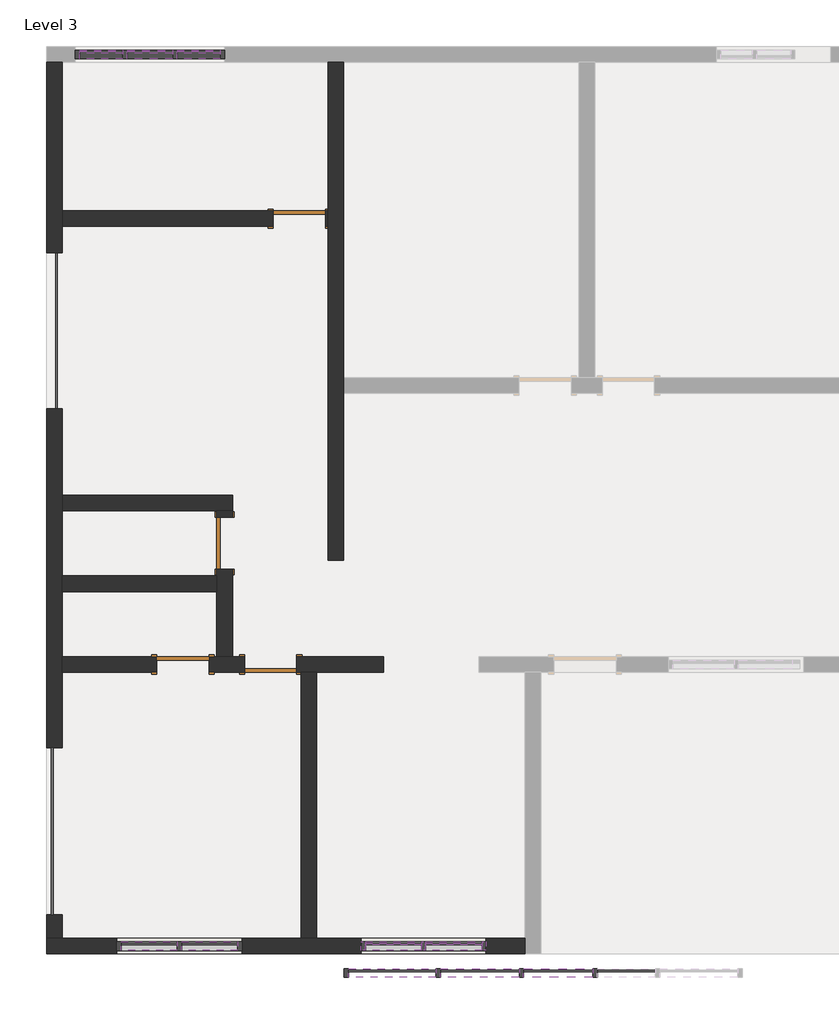
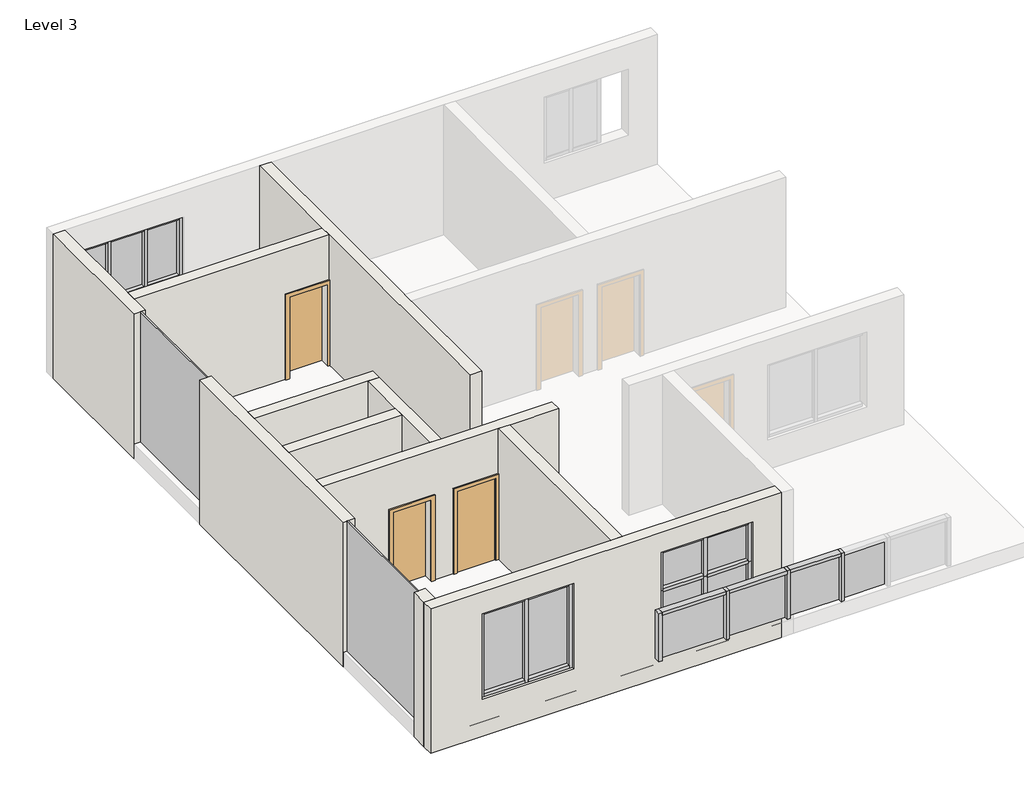
# One storey, part 1 of 2: 36 members, 15 plates, 9 walls, 4 doors.
"""IFC4 building model written with IfcOpenShell, lengths in millimetres."""

from ifc_helpers import new_model, si_unit, frame, origin, place, context, project, spatial, polyline, outline, extrude, faceted_brep, transform, mapped, element, save
from components import door_a1484949, door_85036156, member_c17f1be2, member_ad567e07, member_7f909d8d, member_1a5c3ae3, member_a88312ef, member_3e91fb70, member_7bbb9eab, member_c60babaf, member_5095b95d, member_5a9e6520, member_cba00588, member_d7472725, member_77514b12, member_7dabcdc2, member_870cb0cc, system_panel_glazed_9d4ca976, system_panel_glazed_c60cfc80, system_panel_glazed_61b33e5d, system_panel_glazed_d181f412, system_panel_glazed_8adc4deb, system_panel_glazed_f90b12a9, system_panel_glazed_bf93abc5, system_panel_glazed_f13871fb, system_panel_glazed_bbd5fb98, system_panel_glazed_1e141fc7

model = new_model("IFC4")

# Units and contexts
model_context = context("Model", 3, world=origin())
ifc_project = project(units=[si_unit("LENGTHUNIT", "METRE", prefix="MILLI")], contexts=[model_context])

# Site, building, storey
site = spatial("IfcSite", under=ifc_project)
building = spatial("IfcBuilding", under=site)
storey = spatial("IfcBuildingStorey", under=building, Name="Level 3", Elevation=6096.0)

# Doors
placement = place(None, origin())
door_shape = door_a1484949(model_context)
element("IfcDoor", 1, ObjectType="Single-Flush : 30\" x 80\"", at=placement, inside=storey, context=model_context, shape_type="MappedRepresentation", body=[
    mapped(door_shape, transform((-18291.691855, -9625.0538163, 6096.0), x_axis=(1.0, 0.0, 0.0), y_axis=(0.0, 1.0, 0.0), z_axis=(0.0, 0.0, 1.0))),
])
element("IfcDoor", 2, ObjectType="Single-Flush : 30\" x 80\"", at=placement, inside=storey, context=model_context, shape_type="MappedRepresentation", body=[
    mapped(door_shape, transform((-16589.891855, -3109.9538163, 6096.0), x_axis=(1.0, 0.0, 0.0), y_axis=(0.0, 1.0, 0.0), z_axis=(0.0, 0.0, 1.0))),
])
door_2_shape = door_85036156(model_context)
element("IfcDoor", 3, ObjectType="Single-Flush : 30\" x 80\"", at=placement, inside=storey, context=model_context, shape_type="MappedRepresentation", body=[
    mapped(door_2_shape, transform((-17008.991855, -9625.0538163, 6096.0), x_axis=(1.0, 0.0, 0.0), y_axis=(0.0, 1.0, 0.0), z_axis=(0.0, 0.0, 1.0))),
])
element("IfcDoor", 4, ObjectType="Single-Flush : 30\" x 80\"", at=placement, inside=storey, context=model_context, shape_type="MappedRepresentation", body=[
    mapped(door_2_shape, transform((-17682.091855, -7853.4038163, 6096.0), x_axis=(0.0, -1.0, 0.0), y_axis=(1.0, 0.0, 0.0), z_axis=(0.0, 0.0, 1.0))),
])

# Members
member_shape = member_c17f1be2(model_context)
element("IfcMember", 5, ObjectType="Rectangular Mullion : 2.5\" x 5\" rectangular", at=placement, inside=storey, context=model_context, shape_type="MappedRepresentation", body=[
    mapped(member_shape, transform((-14805.541855, -13739.8538163, 8725.3928177), x_axis=(0.0, 0.0, 1.0), y_axis=(0.0, -1.0, 0.0), z_axis=(1.0, 0.0, 0.0))),
])
element("IfcMember", 6, ObjectType="Rectangular Mullion : 2.5\" x 5\" rectangular", at=placement, inside=storey, context=model_context, shape_type="MappedRepresentation", body=[
    mapped(member_shape, transform((-13922.891855, -13739.8538163, 8725.3928177), x_axis=(0.0, 0.0, 1.0), y_axis=(0.0, -1.0, 0.0), z_axis=(1.0, 0.0, 0.0))),
])
element("IfcMember", 7, ObjectType="Rectangular Mullion : 2.5\" x 5\" rectangular", at=placement, inside=storey, context=model_context, shape_type="MappedRepresentation", body=[
    mapped(member_shape, transform((-18374.241855, -13739.8538163, 8676.8631794), x_axis=(0.0, 0.0, 1.0), y_axis=(0.0, -1.0, 0.0), z_axis=(1.0, 0.0, 0.0))),
])
element("IfcMember", 8, ObjectType="Rectangular Mullion : 2.5\" x 5\" rectangular", at=placement, inside=storey, context=model_context, shape_type="MappedRepresentation", body=[
    mapped(member_shape, transform((-17491.591855, -13739.8538163, 8676.8631794), x_axis=(0.0, 0.0, 1.0), y_axis=(0.0, -1.0, 0.0), z_axis=(1.0, 0.0, 0.0))),
])
member_2_shape = member_ad567e07(model_context)
element("IfcMember", 9, ObjectType="Rectangular Mullion : 2.5\" x 5\" rectangular", at=placement, inside=storey, context=model_context, shape_type="MappedRepresentation", body=[
    mapped(member_2_shape, transform((-13922.891855, -13739.8538163, 7870.5495936), x_axis=(0.0, 0.0, 1.0), y_axis=(0.0, -1.0, 0.0), z_axis=(1.0, 0.0, 0.0))),
])
element("IfcMember", 10, ObjectType="Rectangular Mullion : 2.5\" x 5\" rectangular", at=placement, inside=storey, context=model_context, shape_type="MappedRepresentation", body=[
    mapped(member_2_shape, transform((-14805.541855, -13739.8538163, 7870.5495936), x_axis=(0.0, 0.0, 1.0), y_axis=(0.0, -1.0, 0.0), z_axis=(1.0, 0.0, 0.0))),
])
element("IfcMember", 11, ObjectType="Rectangular Mullion : 2.5\" x 5\" rectangular", at=placement, inside=storey, context=model_context, shape_type="MappedRepresentation", body=[
    mapped(member_shape, transform((-14742.041855, -13739.8538163, 7015.7063696), x_axis=(0.0, 0.0, -1.0), y_axis=(0.0, -1.0, 0.0), z_axis=(-1.0, 0.0, 0.0))),
])
element("IfcMember", 12, ObjectType="Rectangular Mullion : 2.5\" x 5\" rectangular", at=placement, inside=storey, context=model_context, shape_type="MappedRepresentation", body=[
    mapped(member_shape, transform((-15624.691855, -13739.8538163, 7015.7063696), x_axis=(0.0, 0.0, -1.0), y_axis=(0.0, -1.0, 0.0), z_axis=(-1.0, 0.0, 0.0))),
])
element("IfcMember", 13, ObjectType="Rectangular Mullion : 2.5\" x 5\" rectangular", at=placement, inside=storey, context=model_context, shape_type="MappedRepresentation", body=[
    mapped(member_shape, transform((-18310.741855, -13739.8538163, 6875.7032327), x_axis=(0.0, 0.0, -1.0), y_axis=(0.0, -1.0, 0.0), z_axis=(-1.0, 0.0, 0.0))),
])
element("IfcMember", 14, ObjectType="Rectangular Mullion : 2.5\" x 5\" rectangular", at=placement, inside=storey, context=model_context, shape_type="MappedRepresentation", body=[
    mapped(member_shape, transform((-19193.391855, -13739.8538163, 6875.7032327), x_axis=(0.0, 0.0, -1.0), y_axis=(0.0, -1.0, 0.0), z_axis=(-1.0, 0.0, 0.0))),
])
member_3_shape = member_7f909d8d(model_context)
element("IfcMember", 15, ObjectType="Rectangular Mullion : 2.5\" x 5\" rectangular", at=placement, inside=storey, context=model_context, shape_type="MappedRepresentation", body=[
    mapped(member_3_shape, transform((-19170.1085217, -709.6538163, 8591.2496538), x_axis=(0.0, 0.0, 1.0), y_axis=(0.0, -1.0, 0.0), z_axis=(1.0, 0.0, 0.0))),
])
element("IfcMember", 16, ObjectType="Rectangular Mullion : 2.5\" x 5\" rectangular", at=placement, inside=storey, context=model_context, shape_type="MappedRepresentation", body=[
    mapped(member_3_shape, transform((-17745.591855, -709.6538163, 8591.2496538), x_axis=(0.0, 0.0, 1.0), y_axis=(0.0, -1.0, 0.0), z_axis=(1.0, 0.0, 0.0))),
])
member_4_shape = member_1a5c3ae3(model_context)
element("IfcMember", 17, ObjectType="Rectangular Mullion : 2.5\" x 5\" rectangular", at=placement, inside=storey, context=model_context, shape_type="MappedRepresentation", body=[
    mapped(member_4_shape, transform((-18441.9751883, -709.6538163, 8591.2496538), x_axis=(0.0, 0.0, 1.0), y_axis=(0.0, -1.0, 0.0), z_axis=(1.0, 0.0, 0.0))),
])
member_5_shape = member_a88312ef(model_context)
element("IfcMember", 18, ObjectType="Rectangular Mullion : 2.5\" x 5\" rectangular", at=placement, inside=storey, context=model_context, shape_type="MappedRepresentation", body=[
    mapped(member_5_shape, transform((-19138.3585217, -709.6538163, 7292.9915007), x_axis=(1.0, 0.0, 0.0), y_axis=(0.0, -1.0, 0.0), z_axis=(0.0, 0.0, -1.0))),
])
element("IfcMember", 19, ObjectType="Rectangular Mullion : 2.5\" x 5\" rectangular", at=placement, inside=storey, context=model_context, shape_type="MappedRepresentation", body=[
    mapped(member_5_shape, transform((-18410.2251883, -709.6538163, 7292.9915007), x_axis=(1.0, 0.0, 0.0), y_axis=(0.0, -1.0, 0.0), z_axis=(0.0, 0.0, -1.0))),
])
element("IfcMember", 20, ObjectType="Rectangular Mullion : 2.5\" x 5\" rectangular", at=placement, inside=storey, context=model_context, shape_type="MappedRepresentation", body=[
    mapped(member_4_shape, transform((-19106.6085217, -709.6538163, 7292.9915007), x_axis=(0.0, 0.0, -1.0), y_axis=(0.0, -1.0, 0.0), z_axis=(-1.0, 0.0, 0.0))),
])
element("IfcMember", 21, ObjectType="Rectangular Mullion : 2.5\" x 5\" rectangular", at=placement, inside=storey, context=model_context, shape_type="MappedRepresentation", body=[
    mapped(member_3_shape, transform((-18378.4751883, -709.6538163, 7292.9915007), x_axis=(0.0, 0.0, -1.0), y_axis=(0.0, -1.0, 0.0), z_axis=(-1.0, 0.0, 0.0))),
])
element("IfcMember", 22, ObjectType="Rectangular Mullion : 2.5\" x 5\" rectangular", at=placement, inside=storey, context=model_context, shape_type="MappedRepresentation", body=[
    mapped(member_3_shape, transform((-19802.991855, -709.6538163, 7292.9915007), x_axis=(0.0, 0.0, -1.0), y_axis=(0.0, -1.0, 0.0), z_axis=(-1.0, 0.0, 0.0))),
])
member_6_shape = member_3e91fb70(model_context)
element("IfcMember", 23, ObjectType="Rectangular Mullion : 2.5\" x 5\" rectangular", at=placement, inside=storey, context=model_context, shape_type="MappedRepresentation", body=[
    mapped(member_6_shape, transform((-19866.491855, -709.6538163, 8591.2496538), x_axis=(-1.0, 0.0, 0.0), y_axis=(0.0, -1.0, 0.0), z_axis=(0.0, 0.0, 1.0))),
])
element("IfcMember", 24, ObjectType="Rectangular Mullion : 2.5\" x 5\" rectangular", at=placement, inside=storey, context=model_context, shape_type="MappedRepresentation", body=[
    mapped(member_6_shape, transform((-17682.091855, -709.6538163, 7292.9915007), x_axis=(1.0, 0.0, 0.0), y_axis=(0.0, -1.0, 0.0), z_axis=(0.0, 0.0, -1.0))),
])
member_7_shape = member_7bbb9eab(model_context)
element("IfcMember", 25, ObjectType="Rectangular Mullion : 2.5\" x 5\" rectangular", at=placement, inside=storey, context=model_context, shape_type="MappedRepresentation", body=[
    mapped(member_7_shape, transform((-14773.791855, -13739.8538163, 7870.5495936), x_axis=(1.0, 0.0, 0.0), y_axis=(0.0, -1.0, 0.0), z_axis=(0.0, 0.0, -1.0))),
])
member_8_shape = member_c60babaf(model_context)
element("IfcMember", 26, ObjectType="Rectangular Mullion : 2.5\" x 5\" rectangular", at=placement, inside=storey, context=model_context, shape_type="MappedRepresentation", body=[
    mapped(member_8_shape, transform((-15688.191855, -13739.8538163, 8725.3928177), x_axis=(-1.0, 0.0, 0.0), y_axis=(0.0, -1.0, 0.0), z_axis=(0.0, 0.0, 1.0))),
])
element("IfcMember", 27, ObjectType="Rectangular Mullion : 2.5\" x 5\" rectangular", at=placement, inside=storey, context=model_context, shape_type="MappedRepresentation", body=[
    mapped(member_7_shape, transform((-14773.791855, -13739.8538163, 7015.7063696), x_axis=(1.0, 0.0, 0.0), y_axis=(0.0, -1.0, 0.0), z_axis=(0.0, 0.0, -1.0))),
])
element("IfcMember", 28, ObjectType="Rectangular Mullion : 2.5\" x 5\" rectangular", at=placement, inside=storey, context=model_context, shape_type="MappedRepresentation", body=[
    mapped(member_8_shape, transform((-15688.191855, -13739.8538163, 7870.5495936), x_axis=(-1.0, 0.0, 0.0), y_axis=(0.0, -1.0, 0.0), z_axis=(0.0, 0.0, 1.0))),
])
element("IfcMember", 29, ObjectType="Rectangular Mullion : 2.5\" x 5\" rectangular", at=placement, inside=storey, context=model_context, shape_type="MappedRepresentation", body=[
    mapped(member_8_shape, transform((-13859.391855, -13739.8538163, 7870.5495936), x_axis=(1.0, 0.0, 0.0), y_axis=(0.0, -1.0, 0.0), z_axis=(0.0, 0.0, -1.0))),
])
element("IfcMember", 30, ObjectType="Rectangular Mullion : 2.5\" x 5\" rectangular", at=placement, inside=storey, context=model_context, shape_type="MappedRepresentation", body=[
    mapped(member_8_shape, transform((-13859.391855, -13739.8538163, 7015.7063696), x_axis=(1.0, 0.0, 0.0), y_axis=(0.0, -1.0, 0.0), z_axis=(0.0, 0.0, -1.0))),
])
member_9_shape = member_5095b95d(model_context)
element("IfcMember", 31, ObjectType="Rectangular Mullion : 2.5\" x 5\" rectangular", at=placement, inside=storey, context=model_context, shape_type="MappedRepresentation", body=[
    mapped(member_9_shape, transform((-18342.491855, -13739.8538163, 6875.7032327), x_axis=(1.0, 0.0, 0.0), y_axis=(0.0, -1.0, 0.0), z_axis=(0.0, 0.0, -1.0))),
])
member_10_shape = member_5a9e6520(model_context)
element("IfcMember", 32, ObjectType="Rectangular Mullion : 2.5\" x 5\" rectangular", at=placement, inside=storey, context=model_context, shape_type="MappedRepresentation", body=[
    mapped(member_10_shape, transform((-17428.091855, -13739.8538163, 6875.7032327), x_axis=(1.0, 0.0, 0.0), y_axis=(0.0, -1.0, 0.0), z_axis=(0.0, 0.0, -1.0))),
])
element("IfcMember", 33, ObjectType="Rectangular Mullion : 2.5\" x 5\" rectangular", at=placement, inside=storey, context=model_context, shape_type="MappedRepresentation", body=[
    mapped(member_10_shape, transform((-19256.891855, -13739.8538163, 8676.8631794), x_axis=(-1.0, 0.0, 0.0), y_axis=(0.0, -1.0, 0.0), z_axis=(0.0, 0.0, 1.0))),
])
member_11_shape = member_cba00588(model_context)
element("IfcMember", 34, ObjectType="Rectangular Mullion : 2.5\" x 5\" rectangular", at=placement, inside=storey, context=model_context, shape_type="MappedRepresentation", body=[
    mapped(member_11_shape, transform((-14592.3932214, -14133.5538163, 7725.553622), x_axis=(0.0, 0.0, 1.0), y_axis=(0.0, -1.0, 0.0), z_axis=(1.0, 0.0, 0.0))),
])
member_12_shape = member_d7472725(model_context)
element("IfcMember", 35, ObjectType="Rectangular Mullion : 2.5\" x 5\" rectangular", at=placement, inside=storey, context=model_context, shape_type="MappedRepresentation", body=[
    mapped(member_12_shape, transform((-13373.1932214, -14133.5538163, 7725.553622), x_axis=(0.0, 0.0, 1.0), y_axis=(0.0, -1.0, 0.0), z_axis=(1.0, 0.0, 0.0))),
])
member_13_shape = member_77514b12(model_context)
element("IfcMember", 36, ObjectType="Rectangular Mullion : 2.5\" x 5\" rectangular", at=placement, inside=storey, context=model_context, shape_type="MappedRepresentation", body=[
    mapped(member_13_shape, transform((-12297.9265548, -14133.5538163, 7725.553622), x_axis=(0.0, 0.0, 1.0), y_axis=(0.0, -1.0, 0.0), z_axis=(1.0, 0.0, 0.0))),
])
member_14_shape = member_7dabcdc2(model_context)
element("IfcMember", 37, ObjectType="Rectangular Mullion : 2.5\" x 5\" rectangular", at=placement, inside=storey, context=model_context, shape_type="MappedRepresentation", body=[
    mapped(member_14_shape, transform((-14560.6432214, -14133.5538163, 6705.6), x_axis=(1.0, 0.0, 0.0), y_axis=(0.0, -1.0, 0.0), z_axis=(0.0, 0.0, -1.0))),
])
element("IfcMember", 38, ObjectType="Rectangular Mullion : 2.5\" x 5\" rectangular", at=placement, inside=storey, context=model_context, shape_type="MappedRepresentation", body=[
    mapped(member_14_shape, transform((-13341.4432214, -14133.5538163, 6705.6), x_axis=(1.0, 0.0, 0.0), y_axis=(0.0, -1.0, 0.0), z_axis=(0.0, 0.0, -1.0))),
])
element("IfcMember", 39, ObjectType="Rectangular Mullion : 2.5\" x 5\" rectangular", at=placement, inside=storey, context=model_context, shape_type="MappedRepresentation", body=[
    mapped(member_14_shape, transform((-12266.1765548, -14133.5538163, 6705.6), x_axis=(1.0, 0.0, 0.0), y_axis=(0.0, -1.0, 0.0), z_axis=(0.0, 0.0, -1.0))),
])
member_15_shape = member_870cb0cc(model_context)
element("IfcMember", 40, ObjectType="Rectangular Mullion : 2.5\" x 5\" rectangular", at=placement, inside=storey, context=model_context, shape_type="MappedRepresentation", body=[
    mapped(member_15_shape, transform((-15932.2432214, -14133.5538163, 7725.553622), x_axis=(-1.0, 0.0, 0.0), y_axis=(0.0, -1.0, 0.0), z_axis=(0.0, 0.0, 1.0))),
])

# Plates
system_panel_glazed_shape = system_panel_glazed_9d4ca976(model_context)
element("IfcPlate", 41, ObjectType="System Panel : Glazed", at=placement, inside=storey, context=model_context, shape_type="MappedRepresentation", body=[
    mapped(system_panel_glazed_shape, transform((-20171.291855, -4748.2538163, 6096.0), x_axis=(0.0, -1.0, 0.0), y_axis=(1.0, 0.0, 0.0), z_axis=(0.0, 0.0, 1.0))),
])
system_panel_glazed_2_shape = system_panel_glazed_c60cfc80(model_context)
element("IfcPlate", 42, ObjectType="System Panel : Glazed", at=placement, inside=storey, context=model_context, shape_type="MappedRepresentation", body=[
    mapped(system_panel_glazed_2_shape, transform((-20171.291855, -12063.4538163, 6096.0), x_axis=(0.0, 1.0, 0.0), y_axis=(-1.0, 0.0, 0.0), z_axis=(0.0, 0.0, 1.0))),
])
system_panel_glazed_3_shape = system_panel_glazed_61b33e5d(model_context)
element("IfcPlate", 43, ObjectType="System Panel : Glazed", at=placement, inside=storey, context=model_context, shape_type="MappedRepresentation", body=[
    mapped(system_panel_glazed_3_shape, transform((-19486.5501883, -709.6538163, 7356.4915007), x_axis=(1.0, 0.0, 0.0), y_axis=(0.0, 1.0, 0.0), z_axis=(0.0, 0.0, 1.0))),
])
element("IfcPlate", 44, ObjectType="System Panel : Glazed", at=placement, inside=storey, context=model_context, shape_type="MappedRepresentation", body=[
    mapped(system_panel_glazed_3_shape, transform((-18062.0335217, -709.6538163, 7356.4915007), x_axis=(1.0, 0.0, 0.0), y_axis=(0.0, 1.0, 0.0), z_axis=(0.0, 0.0, 1.0))),
])
system_panel_glazed_4_shape = system_panel_glazed_d181f412(model_context)
element("IfcPlate", 45, ObjectType="System Panel : Glazed", at=placement, inside=storey, context=model_context, shape_type="MappedRepresentation", body=[
    mapped(system_panel_glazed_4_shape, transform((-18774.291855, -709.6538163, 7356.4915007), x_axis=(1.0, 0.0, 0.0), y_axis=(0.0, 1.0, 0.0), z_axis=(0.0, 0.0, 1.0))),
])
system_panel_glazed_5_shape = system_panel_glazed_8adc4deb(model_context)
element("IfcPlate", 46, ObjectType="System Panel : Glazed", at=placement, inside=storey, context=model_context, shape_type="MappedRepresentation", body=[
    mapped(system_panel_glazed_5_shape, transform((-15215.116855, -13739.8538163, 7079.2063696), x_axis=(1.0, 0.0, 0.0), y_axis=(0.0, 1.0, 0.0), z_axis=(0.0, 0.0, 1.0))),
])
element("IfcPlate", 47, ObjectType="System Panel : Glazed", at=placement, inside=storey, context=model_context, shape_type="MappedRepresentation", body=[
    mapped(system_panel_glazed_5_shape, transform((-14332.466855, -13739.8538163, 7079.2063696), x_axis=(1.0, 0.0, 0.0), y_axis=(0.0, 1.0, 0.0), z_axis=(0.0, 0.0, 1.0))),
])
element("IfcPlate", 48, ObjectType="System Panel : Glazed", at=placement, inside=storey, context=model_context, shape_type="MappedRepresentation", body=[
    mapped(system_panel_glazed_5_shape, transform((-15215.116855, -13739.8538163, 7902.2995936), x_axis=(1.0, 0.0, 0.0), y_axis=(0.0, 1.0, 0.0), z_axis=(0.0, 0.0, 1.0))),
])
element("IfcPlate", 49, ObjectType="System Panel : Glazed", at=placement, inside=storey, context=model_context, shape_type="MappedRepresentation", body=[
    mapped(system_panel_glazed_5_shape, transform((-14332.466855, -13739.8538163, 7902.2995936), x_axis=(1.0, 0.0, 0.0), y_axis=(0.0, 1.0, 0.0), z_axis=(0.0, 0.0, 1.0))),
])
system_panel_glazed_6_shape = system_panel_glazed_f90b12a9(model_context)
element("IfcPlate", 50, ObjectType="System Panel : Glazed", at=placement, inside=storey, context=model_context, shape_type="MappedRepresentation", body=[
    mapped(system_panel_glazed_6_shape, transform((-18783.816855, -13739.8538163, 6939.2032327), x_axis=(1.0, 0.0, 0.0), y_axis=(0.0, 1.0, 0.0), z_axis=(0.0, 0.0, 1.0))),
])
element("IfcPlate", 51, ObjectType="System Panel : Glazed", at=placement, inside=storey, context=model_context, shape_type="MappedRepresentation", body=[
    mapped(system_panel_glazed_6_shape, transform((-17901.166855, -13739.8538163, 6939.2032327), x_axis=(1.0, 0.0, 0.0), y_axis=(0.0, 1.0, 0.0), z_axis=(0.0, 0.0, 1.0))),
])
system_panel_glazed_7_shape = system_panel_glazed_bf93abc5(model_context)
element("IfcPlate", 52, ObjectType="System Panel : Glazed", at=placement, inside=storey, context=model_context, shape_type="MappedRepresentation", body=[
    mapped(system_panel_glazed_7_shape, transform((-15230.5682214, -14133.5538163, 6705.6), x_axis=(1.0, 0.0, 0.0), y_axis=(0.0, 1.0, 0.0), z_axis=(0.0, 0.0, 1.0))),
])
system_panel_glazed_8_shape = system_panel_glazed_f13871fb(model_context)
element("IfcPlate", 53, ObjectType="System Panel : Glazed", at=placement, inside=storey, context=model_context, shape_type="MappedRepresentation", body=[
    mapped(system_panel_glazed_8_shape, transform((-13951.0432214, -14133.5538163, 6705.6), x_axis=(1.0, 0.0, 0.0), y_axis=(0.0, 1.0, 0.0), z_axis=(0.0, 0.0, 1.0))),
])
system_panel_glazed_9_shape = system_panel_glazed_bbd5fb98(model_context)
element("IfcPlate", 54, ObjectType="System Panel : Glazed", at=placement, inside=storey, context=model_context, shape_type="MappedRepresentation", body=[
    mapped(system_panel_glazed_9_shape, transform((-12803.8098881, -14133.5538163, 6705.6), x_axis=(1.0, 0.0, 0.0), y_axis=(0.0, 1.0, 0.0), z_axis=(0.0, 0.0, 1.0))),
])
system_panel_glazed_10_shape = system_panel_glazed_1e141fc7(model_context)
element("IfcPlate", 55, ObjectType="System Panel : Glazed", at=placement, inside=storey, context=model_context, shape_type="MappedRepresentation", body=[
    mapped(system_panel_glazed_10_shape, transform((-11808.9765548, -14133.5538163, 6705.6), x_axis=(1.0, 0.0, 0.0), y_axis=(0.0, 1.0, 0.0), z_axis=(0.0, 0.0, 1.0))),
])

# Walls
element("IfcWall", 56, ObjectType="9\"", at=placement, inside=storey, context=model_context, shape_type="Brep", body=[
    faceted_brep([(-13287.891855, -13625.5538163, 6096.0), (-16335.891855, -13625.5538163, 6096.0), (-16564.491855, -13625.5538163, 6096.0), (-20056.991855, -13625.5538163, 6096.0), (-20285.591855, -13625.5538163, 6096.0), (-20285.591855, -13625.5538163, 9144.0), (-20056.991855, -13625.5538163, 9144.0), (-16564.491855, -13625.5538163, 9144.0), (-16335.891855, -13625.5538163, 9144.0), (-13287.891855, -13625.5538163, 9144.0), (-15688.191855, -13625.5538163, 8725.3928177), (-15688.191855, -13625.5538163, 7015.7063696), (-13859.391855, -13625.5538163, 7015.7063696), (-13859.391855, -13625.5538163, 8725.3928177), (-19256.891855, -13625.5538163, 8676.8631794), (-19256.891855, -13625.5538163, 6875.7032327), (-17428.091855, -13625.5538163, 6875.7032327), (-17428.091855, -13625.5538163, 8676.8631794), (-20285.591855, -13854.1538163, 6096.0), (-13287.891855, -13854.1538163, 6096.0), (-13287.891855, -13854.1538163, 9144.0), (-20285.591855, -13854.1538163, 9144.0), (-15688.191855, -13854.1538163, 7015.7063696), (-15688.191855, -13854.1538163, 8725.3928177), (-13859.391855, -13854.1538163, 8725.3928177), (-13859.391855, -13854.1538163, 7015.7063696), (-19256.891855, -13854.1538163, 6875.7032327), (-19256.891855, -13854.1538163, 8676.8631794), (-17428.091855, -13854.1538163, 8676.8631794), (-17428.091855, -13854.1538163, 6875.7032327)], [[[0, 1, 2, 3, 4, 5, 6, 7, 8, 9], [10, 11, 12, 13], [14, 15, 16, 17]], [[18, 19, 20, 21], [22, 23, 24, 25], [26, 27, 28, 29]], [[4, 3, 2, 1, 0, 19, 18]], [[9, 8, 7, 6, 5, 21, 20]], [[0, 9, 20, 19]], [[5, 4, 18, 21]], [[10, 23, 22, 11]], [[23, 10, 13, 24]], [[24, 13, 12, 25]], [[11, 22, 25, 12]], [[26, 15, 14, 27]], [[27, 14, 17, 28]], [[28, 17, 16, 29]], [[15, 26, 29, 16]]]),
])
element("IfcWall", 57, ObjectType="9\"", at=placement, inside=storey, context=model_context, shape_type="Brep", body=[
    faceted_brep([(-20056.991855, -13625.5538163, 9144.0), (-20056.991855, -13625.5538163, 6096.0), (-20056.991855, -13282.6538163, 6096.0), (-20056.991855, -13282.6538163, 9144.0), (-20285.591855, -13625.5538163, 6096.0), (-20285.591855, -13625.5538163, 9144.0), (-20285.591855, -13282.6538163, 9144.0), (-20285.591855, -13282.6538163, 6096.0)], [[[0, 1, 2, 3]], [[4, 5, 6, 7]], [[1, 4, 7, 2]], [[5, 0, 3, 6]], [[1, 0, 5, 4]], [[3, 2, 7, 6]]]),
    faceted_brep([(-20056.991855, -823.9538163, 6096.0), (-20056.991855, -823.9538163, 9144.0), (-20056.991855, -2995.6538163, 9144.0), (-20056.991855, -3224.2538163, 9144.0), (-20056.991855, -3605.2538163, 9144.0), (-20056.991855, -3605.2538163, 6096.0), (-20056.991855, -3224.2538163, 6096.0), (-20056.991855, -2995.6538163, 6096.0), (-20285.591855, -823.9538163, 9144.0), (-20285.591855, -823.9538163, 6096.0), (-20285.591855, -3605.2538163, 6096.0), (-20285.591855, -3605.2538163, 9144.0)], [[[0, 1, 2, 3, 4, 5, 6, 7]], [[8, 9, 10, 11]], [[9, 0, 7, 6, 5, 10]], [[1, 8, 11, 4, 3, 2]], [[1, 0, 9, 8]], [[5, 4, 11, 10]]]),
    faceted_brep([(-20056.991855, -5891.2538163, 6096.0), (-20056.991855, -5891.2538163, 9144.0), (-20056.991855, -7148.5538163, 9144.0), (-20056.991855, -7377.1538163, 9144.0), (-20056.991855, -8329.6538163, 9144.0), (-20056.991855, -8558.2538163, 9144.0), (-20056.991855, -9510.7538163, 9144.0), (-20056.991855, -9739.3538163, 9144.0), (-20056.991855, -10844.2538163, 9144.0), (-20056.991855, -10844.2538163, 6096.0), (-20056.991855, -9739.3538163, 6096.0), (-20056.991855, -9510.7538163, 6096.0), (-20056.991855, -8558.2538163, 6096.0), (-20056.991855, -8329.6538163, 6096.0), (-20056.991855, -7377.1538163, 6096.0), (-20056.991855, -7148.5538163, 6096.0), (-20285.591855, -5891.2538163, 9144.0), (-20285.591855, -5891.2538163, 6096.0), (-20285.591855, -10844.2538163, 6096.0), (-20285.591855, -10844.2538163, 9144.0)], [[[0, 1, 2, 3, 4, 5, 6, 7, 8, 9, 10, 11, 12, 13, 14, 15]], [[16, 17, 18, 19]], [[17, 0, 15, 14, 13, 12, 11, 10, 9, 18]], [[1, 16, 19, 8, 7, 6, 5, 4, 3, 2]], [[1, 0, 17, 16]], [[9, 8, 19, 18]]]),
])
element("IfcWall", 58, ObjectType="9\"", at=placement, inside=storey, context=model_context, shape_type="SweptSolid", body=[
    extrude(outline(polyline([(8128.0, -16208.891855), (6096.0, -16208.891855), (6096.0, -16170.791855), (9144.0, -16170.791855), (9144.0, -20056.991855), (6096.0, -20056.991855), (6096.0, -16970.891855), (8128.0, -16970.891855), (8128.0, -16208.891855)])), frame((0.0, -3224.2538163, 0.0), z_axis=(0.0, 1.0, 0.0), x_axis=(0.0, 0.0, 1.0)), (0.0, 0.0, 1.0), 228.6),
])
element("IfcWall", 59, ObjectType="9\"", at=placement, inside=storey, context=model_context, shape_type="Brep", body=[
    faceted_brep([(-15942.191855, -8101.0538163, 6096.0), (-15942.191855, -5662.6538163, 6096.0), (-15942.191855, -5434.0538163, 6096.0), (-15942.191855, -823.9538163, 6096.0), (-15942.191855, -823.9538163, 9144.0), (-15942.191855, -5434.0538163, 9144.0), (-15942.191855, -5662.6538163, 9144.0), (-15942.191855, -8101.0538163, 9144.0), (-16170.791855, -8101.0538163, 6096.0), (-16170.791855, -8101.0538163, 9144.0), (-16170.791855, -3224.2538163, 9144.0), (-16170.791855, -2995.6538163, 9144.0), (-16170.791855, -823.9538163, 9144.0), (-16170.791855, -823.9538163, 6096.0), (-16170.791855, -2995.6538163, 6096.0), (-16170.791855, -3224.2538163, 6096.0)], [[[0, 1, 2, 3, 4, 5, 6, 7]], [[8, 9, 10, 11, 12, 13, 14, 15]], [[3, 2, 1, 0, 8, 15, 14, 13]], [[7, 6, 5, 4, 12, 11, 10, 9]], [[0, 7, 9, 8]], [[4, 3, 13, 12]]]),
])
element("IfcWall", 60, ObjectType="9\"", at=placement, inside=storey, context=model_context, shape_type="SweptSolid", body=[
    extrude(outline(polyline([(-16335.891855, -9739.3538163), (-16335.891855, -13625.5538163), (-16564.491855, -13625.5538163), (-16564.491855, -9739.3538163), (-16335.891855, -9739.3538163)])), frame((0.0, 0.0, 6096.0), z_axis=(0.0, 0.0, 1.0), x_axis=(1.0, 0.0, 0.0)), (0.0, 0.0, 1.0), 3048.0),
])
element("IfcWall", 61, ObjectType="9\"", at=placement, inside=storey, context=model_context, shape_type="Brep", body=[
    faceted_brep([(-17910.691855, -9739.3538163, 8128.0), (-17910.691855, -9739.3538163, 6096.0), (-17389.991855, -9739.3538163, 6096.0), (-17389.991855, -9739.3538163, 8128.0), (-16627.991855, -9739.3538163, 8128.0), (-16627.991855, -9739.3538163, 6096.0), (-16564.491855, -9739.3538163, 6096.0), (-16335.891855, -9739.3538163, 6096.0), (-15357.991855, -9739.3538163, 6096.0), (-15357.991855, -9739.3538163, 9144.0), (-16335.891855, -9739.3538163, 9144.0), (-16564.491855, -9739.3538163, 9144.0), (-20056.991855, -9739.3538163, 9144.0), (-20056.991855, -9739.3538163, 6096.0), (-18672.691855, -9739.3538163, 6096.0), (-18672.691855, -9739.3538163, 8128.0), (-17389.991855, -9510.7538163, 6096.0), (-17567.791855, -9510.7538163, 6096.0), (-17796.391855, -9510.7538163, 6096.0), (-17910.691855, -9510.7538163, 6096.0), (-17910.691855, -9510.7538163, 8128.0), (-18672.691855, -9510.7538163, 8128.0), (-18672.691855, -9510.7538163, 6096.0), (-20056.991855, -9510.7538163, 6096.0), (-20056.991855, -9510.7538163, 9144.0), (-17796.391855, -9510.7538163, 9144.0), (-17567.791855, -9510.7538163, 9144.0), (-15357.991855, -9510.7538163, 9144.0), (-15357.991855, -9510.7538163, 6096.0), (-16627.991855, -9510.7538163, 6096.0), (-16627.991855, -9510.7538163, 8128.0), (-17389.991855, -9510.7538163, 8128.0)], [[[0, 1, 2, 3, 4, 5, 6, 7, 8, 9, 10, 11, 12, 13, 14, 15]], [[16, 17, 18, 19, 20, 21, 22, 23, 24, 25, 26, 27, 28, 29, 30, 31]], [[8, 7, 6, 5, 29, 28]], [[14, 13, 23, 22]], [[2, 1, 19, 18, 17, 16]], [[9, 8, 28, 27]], [[12, 11, 10, 9, 27, 26, 25, 24]], [[13, 12, 24, 23]], [[30, 29, 5, 4]], [[31, 30, 4, 3]], [[16, 31, 3, 2]], [[20, 19, 1, 0]], [[21, 20, 0, 15]], [[22, 21, 15, 14]]]),
])
element("IfcWall", 62, ObjectType="9\"", at=placement, inside=storey, context=model_context, shape_type="Brep", body=[
    faceted_brep([(-20056.991855, -7377.1538163, 6096.0), (-17796.391855, -7377.1538163, 6096.0), (-17567.791855, -7377.1538163, 6096.0), (-17567.791855, -7377.1538163, 9144.0), (-17796.391855, -7377.1538163, 9144.0), (-20056.991855, -7377.1538163, 9144.0), (-20056.991855, -7148.5538163, 6096.0), (-20056.991855, -7148.5538163, 9144.0), (-17567.791855, -7148.5538163, 9144.0), (-17567.791855, -7148.5538163, 6096.0)], [[[0, 1, 2, 3, 4, 5]], [[6, 7, 8, 9]], [[2, 1, 0, 6, 9]], [[5, 4, 3, 8, 7]], [[0, 5, 7, 6]], [[3, 2, 9, 8]]]),
])
element("IfcWall", 63, ObjectType="9\"", at=placement, inside=storey, context=model_context, shape_type="Brep", body=[
    faceted_brep([(-17796.391855, -8234.4038163, 8128.0), (-17796.391855, -8234.4038163, 6096.0), (-17796.391855, -8329.6538163, 6096.0), (-17796.391855, -8558.2538163, 6096.0), (-17796.391855, -9510.7538163, 6096.0), (-17796.391855, -9510.7538163, 9144.0), (-17796.391855, -8558.2538163, 9144.0), (-17796.391855, -8329.6538163, 9144.0), (-17796.391855, -7377.1538163, 9144.0), (-17796.391855, -7377.1538163, 6096.0), (-17796.391855, -7472.4038163, 6096.0), (-17796.391855, -7472.4038163, 8128.0), (-17567.791855, -9510.7538163, 6096.0), (-17567.791855, -8234.4038163, 6096.0), (-17567.791855, -8234.4038163, 8128.0), (-17567.791855, -7472.4038163, 8128.0), (-17567.791855, -7472.4038163, 6096.0), (-17567.791855, -7377.1538163, 6096.0), (-17567.791855, -7377.1538163, 9144.0), (-17567.791855, -9510.7538163, 9144.0)], [[[0, 1, 2, 3, 4, 5, 6, 7, 8, 9, 10, 11]], [[12, 13, 14, 15, 16, 17, 18, 19]], [[10, 9, 17, 16]], [[4, 3, 2, 1, 13, 12]], [[8, 7, 6, 5, 19, 18]], [[9, 8, 18, 17]], [[5, 4, 12, 19]], [[14, 13, 1, 0]], [[15, 14, 0, 11]], [[16, 15, 11, 10]]]),
])
element("IfcWall", 64, ObjectType="9\"", at=placement, inside=storey, context=model_context, shape_type="SweptSolid", body=[
    extrude(outline(polyline([(-20056.991855, -8329.6538163), (-17796.391855, -8329.6538163), (-17796.391855, -8558.2538163), (-20056.991855, -8558.2538163), (-20056.991855, -8329.6538163)])), frame((0.0, 0.0, 6096.0), z_axis=(0.0, 0.0, 1.0), x_axis=(1.0, 0.0, 0.0)), (0.0, 0.0, 1.0), 3048.0),
])

save(model, "model.ifc")

# Revit data of these elements
# Type "Single-Flush : 30\" x 80\""
#   Type Mark = "5"
#   Construction Type Id = "MDOOR"
#   Assembly Code = "C1020"
#   Analytic Construction = "Metal"
#   Thickness = 0' - 2"
#   Heat Transfer Coefficient (U) = 0.651978 BTU/(h·ft²·°F)
#   Height = 6' - 8"
#   Trim Projection Ext = 0' - 1"
#   Trim Projection Int = 0' - 1"
#   Trim Width = 0' - 3"
#   Width = 2' - 6"
#   Define Thermal Properties by = 1
#   Define Thermal Properties by = 1
#   Door Material = Door - Panel
#   Frame Material = Door - Frame
#   Visual Light Transmittance = 0
#   Solar Heat Gain Coefficient = 0
#   Function = (empty or 0)
#   Wall Closure = (empty or 0)
# Type "Rectangular Mullion : 2.5\" x 5\" rectangular"
#   built-in parameter 1007304 = 0.416667 (stored number, unit not read)
#   built-in parameter 1007301 = 0.104167 (stored number, unit not read)
#   built-in parameter 1007300 = 0.104167 (stored number, unit not read)
# Type "System Panel : Glazed"
#   Construction Type Id = "GSP4R"
#   Analytic Construction = "1/8 in Pilkington single glazing"
#   Visual Light Transmittance = 0.9
#   Solar Heat Gain Coefficient = 0.86
#   Heat Transfer Coefficient (U) = 1.18115 BTU/(h·ft²·°F)
#   Define Thermal Properties by = 1
# Type "9\""
#   Assembly Code = "B2010"
#   Layers, outside or top first: 0' - 9" no material (function 1)
# Elements 1, 2, 3, 4 (IfcDoor, "Single-Flush : 30\" x 80\"")
#   Phase Created = New Construction
#   Materials on its faces: "Door - Frame", "Door - Panel"
# Elements 5, 6, 7, 8, 9, 10, 11, 12, 13, 14, 15, 16, 17, 18, 19, 20, 21, 22, 23, 24, 25, 26, 27, 28, 29, 30, 31, 32, 33, 34, 35, 36, 37, 38, 39, 40 (IfcMember, "Rectangular Mullion : 2.5\" x 5\" rectangular")
#   Phase Created = New Construction
#   Materials on its faces: "Aluminum"
# Elements 41, 42, 43, 44, 45, 46, 47, 48, 49, 50, 51, 52, 53, 54, 55 (IfcPlate, "System Panel : Glazed")
#   Phase Created = New Construction
#   Materials on its faces: "Glass"
# Elements 56, 57, 58, 59, 60, 61, 62, 63, 64 (IfcWall, "9\"")
#   Top Offset = 0' - 0"
#   Base Offset = 0' - 0"
#   Unconnected Height = 10' - 0"
#   wall height = 10' - 0"
#   Phase Created = New Construction
#   Base Constraint = Level 3
#   Materials on its faces: "Default Wall"
# Materials
#   "Door - Panel": class "Wood", colour RGB 210 159 95, transparency 0, Cost = 0
#   "Door - Frame": colour RGB 118 70 51, transparency 0, Cost = 0
#   "Aluminum": class "Metal", colour RGB 247 247 247, transparency 0, Description = "Aluminum 6061", Cost = 0
#   "Glass": class "Glass", colour RGB 0 128 192, transparency 0.75, Description = "Soda Lime Glass", Cost = 0
#   "Default Wall": colour RGB 128 128 128, transparency 0, Cost = 0
